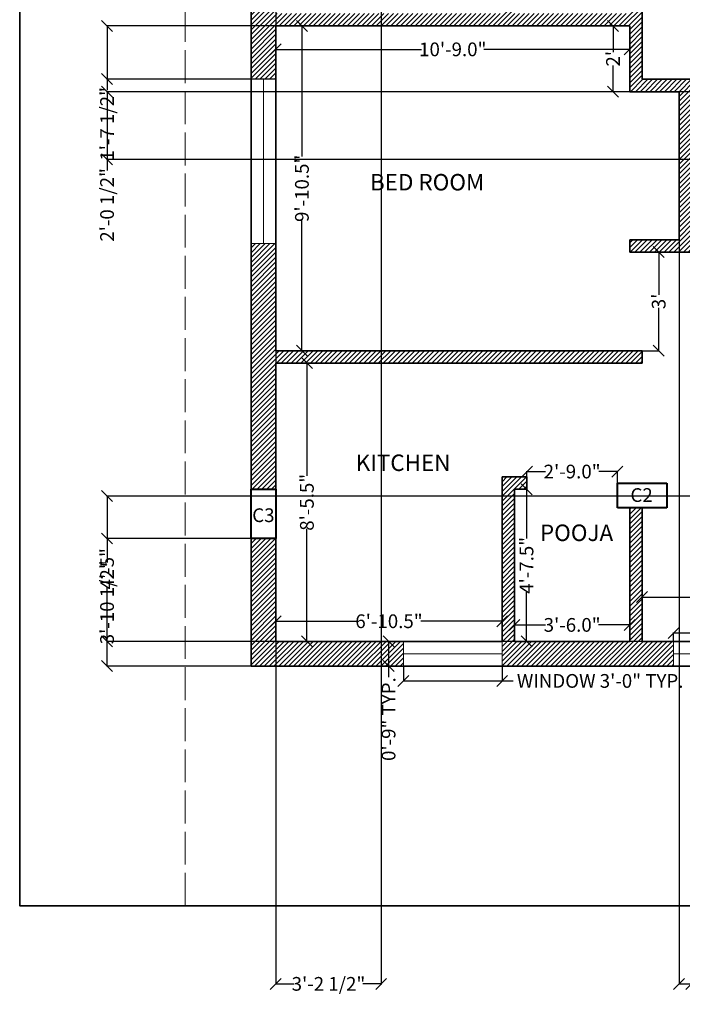
# Model space of a CAD drawing. Units: inches. Extents: x 72 to 538, y -43 to 598.
# Tile 1 of 4: x 72 to 314, y -43 to 316. Entities that reach past the tile are written whole.
import ezdxf

# ---------------------------------------------------------------- set-up
doc = ezdxf.new("R2010")
doc.units = ezdxf.units.IN
doc.header["$MEASUREMENT"] = 0
doc.linetypes.add('ACAD_ISO02W100', pattern=[15, 12, -3])
for name, color, linetype, lineweight in [('A-ANNO-DIMS', 2, 'Continuous', 18), ('A-ANNO-TEXT', 6, 'Continuous', 18), ('A-ANNO-TTLB', 7, 'Continuous', 35), ('A-AREA-IDEN', 7, 'Continuous', 25), ('A-COLS', 6, 'Continuous', 40), ('A-GLAZ', 4, 'Continuous', 18), ('A-WALL', 7, 'Continuous', 35), ('C-PROP', 3, 'ACAD_ISO02W100', 18)]:
    doc.layers.add(name, color=color, linetype=linetype, lineweight=lineweight)
doc.layers.add('A-WALL-PATT', color=30, linetype='Continuous', lineweight=13, true_color=0xf26722)
doc.styles.get("Standard").update_dxf_attribs({"font": 'arial.ttf'})
doc.dimstyles.get("Standard").update_dxf_attribs({"dimtxt": 5, "dimasz": 4, "dimexe": 0.18, "dimexo": 0.0625, "dimgap": 0.09, "dimtad": 0, "dimdec": 1, "dimzin": 0, "dimdsep": 46, "dimlunit": 3, "dimtxsty": 'Standard', "dimblk": 'OBLIQUE', "dimcen": 0.09, "dimadec": 0, "dimazin": 0, "dimtfac": 1, "dimtdec": 1, "dimtofl": 0, "dimtmove": 0, "dimatfit": 3, "dimfxl": 1, "dimtolj": 1, "dimtzin": 0, "dimarcsym": 0})

# ---------------------------------------------------------------- blocks, each defined once
blk = doc.blocks.new('_Oblique')
at = {"color": 0, "linetype": 'ByBlock', "lineweight": -2}
blk.add_line((-0.5, -0.5), (0.5, 0.5), dxfattribs=at)
blk = doc.blocks.new('*D11')
at = {"layer": 'A-ANNO-DIMS', "color": 0, "lineweight": -2, "transparency": 16777216}
for p, q in [((165.63, 313.56), (165.63, 304.87)), ((294.63, 313.56), (294.63, 304.87)), ((165.63, 305.05), (218.77, 305.05)), ((294.63, 305.05), (241.48, 305.05))]:
    blk.add_line(p, q, dxfattribs=at)
at = {"layer": 'Defpoints', "color": 0, "transparency": 16777216}
for p in [(165.63, 313.62), (294.63, 313.62), (294.63, 305.05)]:
    blk.add_point(p, dxfattribs=at)
at = {"layer": 'A-ANNO-DIMS', "color": 0, "lineweight": -2, "transparency": 16777216, "xscale": 4, "yscale": 4, "zscale": 4, "rotation": 180}
blk.add_blockref('_Oblique', (165.63, 305.05), dxfattribs=at)
at = {"layer": 'A-ANNO-DIMS', "color": 0, "lineweight": -2, "transparency": 16777216, "xscale": 4, "yscale": 4, "zscale": 4}
blk.add_blockref('_Oblique', (294.63, 305.05), dxfattribs=at)
at = {"layer": 'A-ANNO-DIMS', "color": 0, "transparency": 16777216, "insert": (230.13, 305.05), "char_height": 5, "attachment_point": 5}
blk.add_mtext('\\A1;10\'-9.0"', dxfattribs=at)
blk = doc.blocks.new('*D12')
at = {"layer": 'A-ANNO-DIMS', "color": 0, "lineweight": -2, "transparency": 16777216}
for p, q in [((294.57, 313.62), (288.36, 313.62)), ((288.54, 313.62), (288.54, 304.05)), ((288.54, 289.62), (288.54, 299.19)), ((294.57, 289.62), (288.36, 289.62))]:
    blk.add_line(p, q, dxfattribs=at)
at = {"layer": 'Defpoints', "color": 0, "transparency": 16777216}
for p in [(294.63, 313.62), (288.54, 289.62), (294.63, 289.62)]:
    blk.add_point(p, dxfattribs=at)
at = {"layer": 'A-ANNO-DIMS', "color": 0, "lineweight": -2, "transparency": 16777216, "xscale": 4, "yscale": 4, "zscale": 4}
for p, rotation in [((288.54, 313.62), 90), ((288.54, 289.62), 270)]:
    blk.add_blockref('_Oblique', p, dxfattribs=dict(at, rotation=rotation))
at = {"layer": 'A-ANNO-DIMS', "color": 0, "transparency": 16777216, "insert": (288.54, 301.62), "char_height": 5, "attachment_point": 5, "rotation": 90}
blk.add_mtext("\\A1;2'", dxfattribs=at)
blk = doc.blocks.new('*D13')
at = {"layer": 'A-ANNO-DIMS', "color": 0, "lineweight": -2, "transparency": 16777216}
for p, q in [((165.69, 313.62), (175.32, 313.62)), ((175.14, 313.62), (175.14, 265.96)), ((175.14, 195.12), (175.14, 242.78)), ((165.69, 195.12), (175.32, 195.12))]:
    blk.add_line(p, q, dxfattribs=at)
at = {"layer": 'Defpoints', "color": 0, "transparency": 16777216}
for p in [(165.63, 313.62), (165.63, 195.12), (175.14, 195.12)]:
    blk.add_point(p, dxfattribs=at)
at = {"layer": 'A-ANNO-DIMS', "color": 0, "lineweight": -2, "transparency": 16777216, "xscale": 4, "yscale": 4, "zscale": 4}
for p, rotation in [((175.14, 313.62), 90), ((175.14, 195.12), 270)]:
    blk.add_blockref('_Oblique', p, dxfattribs=dict(at, rotation=rotation))
at = {"layer": 'A-ANNO-DIMS', "color": 0, "transparency": 16777216, "insert": (175.14, 254.37), "char_height": 5, "attachment_point": 5, "rotation": 90}
blk.add_mtext('\\A1;9\'-10.5"', dxfattribs=at)
blk = doc.blocks.new('*D14')
at = {"layer": 'A-ANNO-DIMS', "color": 0, "lineweight": -2, "transparency": 16777216}
for p, q in [((165.69, 190.62), (177.14, 190.62)), ((176.96, 190.62), (176.96, 149.52)), ((176.96, 89.12), (176.96, 130.22)), ((165.69, 89.12), (177.14, 89.12))]:
    blk.add_line(p, q, dxfattribs=at)
at = {"layer": 'Defpoints', "color": 0, "transparency": 16777216}
for p in [(165.63, 190.62), (165.63, 89.12), (176.96, 89.12)]:
    blk.add_point(p, dxfattribs=at)
at = {"layer": 'A-ANNO-DIMS', "color": 0, "lineweight": -2, "transparency": 16777216, "xscale": 4, "yscale": 4, "zscale": 4}
for p, rotation in [((176.96, 190.62), 90), ((176.96, 89.12), 270)]:
    blk.add_blockref('_Oblique', p, dxfattribs=dict(at, rotation=rotation))
at = {"layer": 'A-ANNO-DIMS', "color": 0, "transparency": 16777216, "insert": (176.96, 139.87), "char_height": 5, "attachment_point": 5, "rotation": 90}
blk.add_mtext('\\A1;8\'-5.5"', dxfattribs=at)
blk = doc.blocks.new('*D15')
at = {"layer": 'A-ANNO-DIMS', "color": 0, "lineweight": -2, "transparency": 16777216}
for p, q in [((165.63, 89.18), (165.63, 96.67)), ((165.63, 96.49), (195.28, 96.49)), ((248.13, 96.49), (218.48, 96.49)), ((248.13, 89.18), (248.13, 96.67))]:
    blk.add_line(p, q, dxfattribs=at)
at = {"layer": 'Defpoints', "color": 0, "transparency": 16777216}
for p in [(248.13, 96.49), (165.63, 89.12), (248.13, 89.12)]:
    blk.add_point(p, dxfattribs=at)
at = {"layer": 'A-ANNO-DIMS', "color": 0, "lineweight": -2, "transparency": 16777216, "xscale": 4, "yscale": 4, "zscale": 4, "rotation": 180}
blk.add_blockref('_Oblique', (165.63, 96.49), dxfattribs=at)
at = {"layer": 'A-ANNO-DIMS', "color": 0, "lineweight": -2, "transparency": 16777216, "xscale": 4, "yscale": 4, "zscale": 4}
blk.add_blockref('_Oblique', (248.13, 96.49), dxfattribs=at)
at = {"layer": 'A-ANNO-DIMS', "color": 0, "transparency": 16777216, "insert": (206.88, 96.49), "char_height": 5, "attachment_point": 5}
blk.add_mtext('\\A1;6\'-10.5"', dxfattribs=at)
blk = doc.blocks.new('*D16')
at = {"layer": 'A-ANNO-DIMS', "color": 0, "lineweight": -2, "transparency": 16777216}
for p, q in [((252.63, 89.18), (252.63, 95.33)), ((252.63, 95.15), (263.98, 95.15)), ((294.63, 95.15), (283.28, 95.15)), ((294.63, 89.18), (294.63, 95.33))]:
    blk.add_line(p, q, dxfattribs=at)
at = {"layer": 'Defpoints', "color": 0, "transparency": 16777216}
for p in [(294.63, 95.15), (252.63, 89.12), (294.63, 89.12)]:
    blk.add_point(p, dxfattribs=at)
at = {"layer": 'A-ANNO-DIMS', "color": 0, "lineweight": -2, "transparency": 16777216, "xscale": 4, "yscale": 4, "zscale": 4, "rotation": 180}
blk.add_blockref('_Oblique', (252.63, 95.15), dxfattribs=at)
at = {"layer": 'A-ANNO-DIMS', "color": 0, "lineweight": -2, "transparency": 16777216, "xscale": 4, "yscale": 4, "zscale": 4}
blk.add_blockref('_Oblique', (294.63, 95.15), dxfattribs=at)
at = {"layer": 'A-ANNO-DIMS', "color": 0, "transparency": 16777216, "insert": (273.63, 95.15), "char_height": 5, "attachment_point": 5}
blk.add_mtext('\\A1;3\'-6.0"', dxfattribs=at)
blk = doc.blocks.new('*D17')
at = {"layer": 'A-ANNO-DIMS', "color": 0, "lineweight": -2, "transparency": 16777216}
for p, q in [((252.69, 144.62), (257.19, 144.62)), ((257.01, 144.62), (257.01, 126.62)), ((257.01, 89.12), (257.01, 107.12)), ((252.69, 89.12), (257.19, 89.12))]:
    blk.add_line(p, q, dxfattribs=at)
at = {"layer": 'Defpoints', "color": 0, "transparency": 16777216}
for p in [(252.63, 144.62), (252.63, 89.12), (257.01, 89.12)]:
    blk.add_point(p, dxfattribs=at)
at = {"layer": 'A-ANNO-DIMS', "color": 0, "lineweight": -2, "transparency": 16777216, "xscale": 4, "yscale": 4, "zscale": 4}
for p, rotation in [((257.01, 144.62), 90), ((257.01, 89.12), 270)]:
    blk.add_blockref('_Oblique', p, dxfattribs=dict(at, rotation=rotation))
at = {"layer": 'A-ANNO-DIMS', "color": 0, "transparency": 16777216, "insert": (257.01, 116.87), "char_height": 5, "attachment_point": 5, "rotation": 90}
blk.add_mtext('\\A1;4\'-7.5"', dxfattribs=at)
blk = doc.blocks.new('*D18')
at = {"layer": 'A-ANNO-DIMS', "color": 0, "lineweight": -2, "transparency": 16777216}
for p, q in [((257.13, 146.93), (257.13, 151.26)), ((257.13, 151.08), (263.94, 151.08)), ((290.13, 151.08), (283.32, 151.08)), ((290.13, 146.93), (290.13, 151.26))]:
    blk.add_line(p, q, dxfattribs=at)
at = {"layer": 'Defpoints', "color": 0, "transparency": 16777216}
for p in [(290.13, 151.08), (257.13, 146.87), (290.13, 146.87)]:
    blk.add_point(p, dxfattribs=at)
at = {"layer": 'A-ANNO-DIMS', "color": 0, "lineweight": -2, "transparency": 16777216, "xscale": 4, "yscale": 4, "zscale": 4, "rotation": 180}
blk.add_blockref('_Oblique', (257.13, 151.08), dxfattribs=at)
at = {"layer": 'A-ANNO-DIMS', "color": 0, "lineweight": -2, "transparency": 16777216, "xscale": 4, "yscale": 4, "zscale": 4}
blk.add_blockref('_Oblique', (290.13, 151.08), dxfattribs=at)
at = {"layer": 'A-ANNO-DIMS', "color": 0, "transparency": 16777216, "insert": (273.63, 151.08), "char_height": 5, "attachment_point": 5}
blk.add_mtext('\\A1;2\'-9.0"', dxfattribs=at)
blk = doc.blocks.new('*D19')
at = {"layer": 'A-ANNO-DIMS', "color": 0, "lineweight": -2, "transparency": 16777216}
for p, q in [((299.19, 231.12), (305.36, 231.12)), ((305.18, 231.12), (305.18, 215.51)), ((305.18, 195.12), (305.18, 210.73)), ((299.19, 195.12), (305.36, 195.12))]:
    blk.add_line(p, q, dxfattribs=at)
at = {"layer": 'Defpoints', "color": 0, "transparency": 16777216}
for p in [(299.13, 231.12), (305.18, 231.12), (299.13, 195.12)]:
    blk.add_point(p, dxfattribs=at)
at = {"layer": 'A-ANNO-DIMS', "color": 0, "lineweight": -2, "transparency": 16777216, "xscale": 4, "yscale": 4, "zscale": 4}
for p, rotation in [((305.18, 231.12), 90), ((305.18, 195.12), 270)]:
    blk.add_blockref('_Oblique', p, dxfattribs=dict(at, rotation=rotation))
at = {"layer": 'A-ANNO-DIMS', "color": 0, "transparency": 16777216, "insert": (305.18, 213.12), "char_height": 5, "attachment_point": 5, "rotation": 90}
blk.add_mtext("\\A1;3'", dxfattribs=at)
blk = doc.blocks.new('*D21')
at = {"layer": 'A-ANNO-DIMS', "color": 0, "lineweight": -2, "transparency": 16777216}
for p, q in [((299.13, 113.52), (299.13, 105.13)), ((441.63, 113.52), (441.63, 105.13)), ((299.13, 105.31), (357.08, 105.31)), ((441.63, 105.31), (383.68, 105.31))]:
    blk.add_line(p, q, dxfattribs=at)
at = {"layer": 'Defpoints', "color": 0, "transparency": 16777216}
for p in [(299.13, 113.59), (441.63, 113.59), (441.63, 105.31)]:
    blk.add_point(p, dxfattribs=at)
at = {"layer": 'A-ANNO-DIMS', "color": 0, "lineweight": -2, "transparency": 16777216, "xscale": 4, "yscale": 4, "zscale": 4, "rotation": 180}
blk.add_blockref('_Oblique', (299.13, 105.31), dxfattribs=at)
at = {"layer": 'A-ANNO-DIMS', "color": 0, "lineweight": -2, "transparency": 16777216, "xscale": 4, "yscale": 4, "zscale": 4}
blk.add_blockref('_Oblique', (441.63, 105.31), dxfattribs=at)
at = {"layer": 'A-ANNO-DIMS', "color": 0, "transparency": 16777216, "insert": (370.38, 105.31), "char_height": 5, "attachment_point": 5}
blk.add_mtext('\\A1;11\'-10.5"', dxfattribs=at)
blk = doc.blocks.new('*D36')
at = {"layer": 'A-ANNO-DIMS', "color": 0, "lineweight": -2, "transparency": 16777216}
for p, q in [((310.61, 89.18), (310.61, 92.39)), ((310.61, 92.21), (338.22, 92.21)), ((370.61, 92.21), (343, 92.21)), ((370.61, 89.18), (370.61, 92.39))]:
    blk.add_line(p, q, dxfattribs=at)
at = {"layer": 'Defpoints', "color": 0, "transparency": 16777216}
for p in [(370.61, 92.21), (310.61, 89.12), (370.61, 89.12)]:
    blk.add_point(p, dxfattribs=at)
at = {"layer": 'A-ANNO-DIMS', "color": 0, "lineweight": -2, "transparency": 16777216, "xscale": 4, "yscale": 4, "zscale": 4, "rotation": 180}
blk.add_blockref('_Oblique', (310.61, 92.21), dxfattribs=at)
at = {"layer": 'A-ANNO-DIMS', "color": 0, "lineweight": -2, "transparency": 16777216, "xscale": 4, "yscale": 4, "zscale": 4}
blk.add_blockref('_Oblique', (370.61, 92.21), dxfattribs=at)
at = {"layer": 'A-ANNO-DIMS', "color": 0, "transparency": 16777216, "insert": (340.61, 92.21), "char_height": 5, "attachment_point": 5}
blk.add_mtext("\\A1;5'", dxfattribs=at)
blk = doc.blocks.new('COL-9X18')
for p, q in [((0, 18), (9, 18)), ((0, 0), (0, 18)), ((9, 18), (9, 0)), ((9, 0), (0, 0))]:
    blk.add_line(p, q)
blk = doc.blocks.new('WIN-60')
for p, q in [((0, 9), (0, 0)), ((60, 9), (60, 0)), ((0, 4.5), (60, 4.5))]:
    blk.add_line(p, q)
blk = doc.blocks.new('WIN-36')
for p, q in [((9, 36), (0, 36)), ((4.5, 36), (4.5, 0)), ((9, 0), (0, 0))]:
    blk.add_line(p, q)
blk = doc.blocks.new('*D48')
at = {"layer": 'A-ANNO-DIMS', "color": 0, "lineweight": -2, "transparency": 16777216}
for p, q in [((212.13, 80.06), (212.13, 74.54)), ((248.13, 80.06), (248.13, 74.54)), ((212.13, 74.72), (248.13, 74.72)), ((248.13, 74.72), (252.13, 74.72))]:
    blk.add_line(p, q, dxfattribs=at)
at = {"layer": 'Defpoints', "color": 0, "transparency": 16777216}
for p in [(212.13, 80.12), (248.13, 80.12), (248.13, 74.72)]:
    blk.add_point(p, dxfattribs=at)
at = {"layer": 'A-ANNO-DIMS', "color": 0, "lineweight": -2, "transparency": 16777216, "xscale": 4, "yscale": 4, "zscale": 4, "rotation": 180}
blk.add_blockref('_Oblique', (212.13, 74.72), dxfattribs=at)
at = {"layer": 'A-ANNO-DIMS', "color": 0, "lineweight": -2, "transparency": 16777216, "xscale": 4, "yscale": 4, "zscale": 4}
blk.add_blockref('_Oblique', (248.13, 74.72), dxfattribs=at)
at = {"layer": 'A-ANNO-DIMS', "color": 0, "transparency": 16777216, "insert": (283.85, 74.72), "char_height": 5, "attachment_point": 5}
blk.add_mtext('\\A1;WINDOW 3\'-0" TYP.', dxfattribs=at)
blk = doc.blocks.new('*D49')
at = {"layer": 'A-ANNO-DIMS', "color": 0, "lineweight": -2, "transparency": 16777216}
for p, q in [((212.07, 89.12), (206.55, 89.12)), ((206.73, 89.12), (206.73, 80.12)), ((212.07, 80.12), (206.55, 80.12)), ((206.73, 80.12), (206.73, 76.12))]:
    blk.add_line(p, q, dxfattribs=at)
at = {"layer": 'Defpoints', "color": 0, "transparency": 16777216}
for p in [(212.13, 89.12), (206.73, 80.12), (212.13, 80.12)]:
    blk.add_point(p, dxfattribs=at)
at = {"layer": 'A-ANNO-DIMS', "color": 0, "lineweight": -2, "transparency": 16777216, "xscale": 4, "yscale": 4, "zscale": 4}
for p, rotation in [((206.73, 89.12), 90), ((206.73, 80.12), 270)]:
    blk.add_blockref('_Oblique', p, dxfattribs=dict(at, rotation=rotation))
at = {"layer": 'A-ANNO-DIMS', "color": 0, "transparency": 16777216, "insert": (206.73, 60.79), "char_height": 5, "attachment_point": 5, "rotation": 90}
blk.add_mtext('\\A1;0\'-9" TYP.', dxfattribs=at)
blk = doc.blocks.new('*D57')
at = {"layer": 'A-ANNO-DIMS', "color": 0, "lineweight": -2, "transparency": 16777216}
for p, q in [((165.63, 527.06), (165.63, -35.94)), ((204.03, 527.06), (204.03, -35.94)), ((165.63, -35.76), (172.27, -35.76)), ((204.03, -35.76), (197.39, -35.76))]:
    blk.add_line(p, q, dxfattribs=at)
at = {"layer": 'Defpoints', "color": 0, "transparency": 16777216}
for p in [(165.63, 527.12), (204.03, 527.12), (204.03, -35.76)]:
    blk.add_point(p, dxfattribs=at)
at = {"layer": 'A-ANNO-DIMS', "color": 0, "lineweight": -2, "transparency": 16777216, "xscale": 4, "yscale": 4, "zscale": 4, "rotation": 180}
blk.add_blockref('_Oblique', (165.63, -35.76), dxfattribs=at)
at = {"layer": 'A-ANNO-DIMS', "color": 0, "lineweight": -2, "transparency": 16777216, "xscale": 4, "yscale": 4, "zscale": 4}
blk.add_blockref('_Oblique', (204.03, -35.76), dxfattribs=at)
at = {"layer": 'A-ANNO-DIMS', "color": 0, "transparency": 16777216, "insert": (184.83, -35.76), "char_height": 5, "attachment_point": 5}
blk.add_mtext('\\A1;3\'-2 1/2"', dxfattribs=at)
blk = doc.blocks.new('*D59')
at = {"layer": 'A-ANNO-DIMS', "color": 0, "lineweight": -2, "transparency": 16777216}
for p, q in [((165.57, 313.62), (103.95, 313.62)), ((104.13, 313.62), (104.13, 294.2)), ((165.57, 294.2), (103.95, 294.2)), ((104.13, 294.2), (104.13, 290.2))]:
    blk.add_line(p, q, dxfattribs=at)
at = {"layer": 'Defpoints', "color": 0, "transparency": 16777216}
for p in [(165.63, 313.62), (104.13, 294.2), (165.63, 294.2)]:
    blk.add_point(p, dxfattribs=at)
at = {"layer": 'A-ANNO-DIMS', "color": 0, "lineweight": -2, "transparency": 16777216, "xscale": 4, "yscale": 4, "zscale": 4}
for p, rotation in [((104.13, 313.62), 90), ((104.13, 294.2), 270)]:
    blk.add_blockref('_Oblique', p, dxfattribs=dict(at, rotation=rotation))
at = {"layer": 'A-ANNO-DIMS', "color": 0, "transparency": 16777216, "insert": (104.13, 277.88), "char_height": 5, "attachment_point": 5, "rotation": 90}
blk.add_mtext('\\A1;1\'-7 1/2"', dxfattribs=at)
blk = doc.blocks.new('*D65')
at = {"layer": 'A-ANNO-DIMS', "color": 0, "lineweight": -2, "transparency": 16777216}
for p, q in [((312.63, 235.56), (312.63, -35.94)), ((317.13, 231.06), (317.13, -35.94)), ((312.63, -35.76), (317.13, -35.76)), ((317.13, -35.76), (321.13, -35.76))]:
    blk.add_line(p, q, dxfattribs=at)
at = {"layer": 'Defpoints', "color": 0, "transparency": 16777216}
for p in [(312.63, 235.62), (317.13, 231.12), (317.13, -35.76)]:
    blk.add_point(p, dxfattribs=at)
at = {"layer": 'A-ANNO-DIMS', "color": 0, "lineweight": -2, "transparency": 16777216, "xscale": 4, "yscale": 4, "zscale": 4, "rotation": 180}
blk.add_blockref('_Oblique', (312.63, -35.76), dxfattribs=at)
at = {"layer": 'A-ANNO-DIMS', "color": 0, "lineweight": -2, "transparency": 16777216, "xscale": 4, "yscale": 4, "zscale": 4}
blk.add_blockref('_Oblique', (317.13, -35.76), dxfattribs=at)
at = {"layer": 'A-ANNO-DIMS', "color": 0, "transparency": 16777216, "insert": (333.69, -35.76), "char_height": 5, "attachment_point": 5}
blk.add_mtext('\\A1;0\'-4 1/2"', dxfattribs=at)
blk = doc.blocks.new('*D66')
at = {"layer": 'A-ANNO-DIMS', "color": 0, "lineweight": -2, "transparency": 16777216}
for p, q in [((441.57, 289.62), (103.95, 289.62)), ((104.13, 289.62), (104.13, 264.93)), ((441.57, 264.93), (103.95, 264.93)), ((104.13, 264.93), (104.13, 260.93))]:
    blk.add_line(p, q, dxfattribs=at)
at = {"layer": 'Defpoints', "color": 0, "transparency": 16777216}
for p in [(441.63, 289.62), (104.13, 264.93), (441.63, 264.93)]:
    blk.add_point(p, dxfattribs=at)
at = {"layer": 'A-ANNO-DIMS', "color": 0, "lineweight": -2, "transparency": 16777216, "xscale": 4, "yscale": 4, "zscale": 4}
for p, rotation in [((104.13, 289.62), 90), ((104.13, 264.93), 270)]:
    blk.add_blockref('_Oblique', p, dxfattribs=dict(at, rotation=rotation))
at = {"layer": 'A-ANNO-DIMS', "color": 0, "transparency": 16777216, "insert": (104.13, 248.33), "char_height": 5, "attachment_point": 5, "rotation": 90}
blk.add_mtext('\\A1;2\'-0 1/2"', dxfattribs=at)
blk = doc.blocks.new('*D67')
at = {"layer": 'A-ANNO-DIMS', "color": 0, "lineweight": -2, "transparency": 16777216}
for p, q in [((156.57, 126.66), (103.95, 126.66)), ((104.13, 126.66), (104.13, 117.89)), ((104.13, 80.12), (104.13, 88.89)), ((156.57, 80.12), (103.95, 80.12))]:
    blk.add_line(p, q, dxfattribs=at)
at = {"layer": 'Defpoints', "color": 0, "transparency": 16777216}
for p in [(156.63, 126.66), (104.13, 80.12), (156.63, 80.12)]:
    blk.add_point(p, dxfattribs=at)
at = {"layer": 'A-ANNO-DIMS', "color": 0, "lineweight": -2, "transparency": 16777216, "xscale": 4, "yscale": 4, "zscale": 4}
for p, rotation in [((104.13, 126.66), 90), ((104.13, 80.12), 270)]:
    blk.add_blockref('_Oblique', p, dxfattribs=dict(at, rotation=rotation))
at = {"layer": 'A-ANNO-DIMS', "color": 0, "transparency": 16777216, "insert": (104.13, 103.39), "char_height": 5, "attachment_point": 5, "rotation": 90}
blk.add_mtext('\\A1;3\'-10 1/2"', dxfattribs=at)
blk = doc.blocks.new('*D69')
at = {"layer": 'A-ANNO-DIMS', "color": 0, "lineweight": -2, "transparency": 16777216}
for p, q in [((441.57, 142.12), (103.95, 142.12)), ((104.13, 142.12), (104.13, 122.46)), ((104.13, 89.12), (104.13, 108.78)), ((441.57, 89.12), (103.95, 89.12))]:
    blk.add_line(p, q, dxfattribs=at)
at = {"layer": 'Defpoints', "color": 0, "transparency": 16777216}
for p in [(441.63, 142.12), (104.13, 89.12), (441.63, 89.12)]:
    blk.add_point(p, dxfattribs=at)
at = {"layer": 'A-ANNO-DIMS', "color": 0, "lineweight": -2, "transparency": 16777216, "xscale": 4, "yscale": 4, "zscale": 4}
for p, rotation in [((104.13, 142.12), 90), ((104.13, 89.12), 270)]:
    blk.add_blockref('_Oblique', p, dxfattribs=dict(at, rotation=rotation))
at = {"layer": 'A-ANNO-DIMS', "color": 0, "transparency": 16777216, "insert": (104.13, 115.62), "char_height": 5, "attachment_point": 5, "rotation": 90}
blk.add_mtext('\\A1;4\'-5"', dxfattribs=at)

msp = doc.modelspace()

# ---------------------------------------------------------------- hatches: boundary and pattern name
at = {"layer": 'A-WALL-PATT'}
h = msp.add_hatch(dxfattribs=at)
h.set_pattern_fill('ANSI31', color=256, scale=10)
h.paths.add_polyline_path([(204.03, 536.12), (165.63, 536.12), (165.63, 527.12), (204.03, 527.12)])
h.paths.add_polyline_path([(165.63, 487.18), (165.63, 518.12), (156.63, 518.12), (156.63, 487.18)])
h.paths.add_polyline_path([(374.85, 253.74), (416.04, 253.74), (416.04, 266.11), (374.85, 266.11)], flags=9)
h.paths.add_polyline_path([(358.05, 165.41), (382.02, 165.41), (382.02, 177.78), (358.05, 177.78)], flags=9)
h.paths.add_polyline_path([(258.82, 340.82), (290.25, 340.82), (290.25, 353.18), (258.82, 353.18)], flags=9)
h.paths.add_polyline_path([(190.8, 385.39), (230.59, 385.39), (230.59, 397.75), (190.8, 397.75)], flags=9)
h.paths.add_polyline_path([(259.76, 122.35), (291.18, 122.35), (291.18, 134.72), (259.76, 134.72)], flags=9)
h.paths.add_polyline_path([(192.66, 147.9), (232.45, 147.9), (232.45, 160.26), (192.66, 160.26)], flags=9)
h.paths.add_polyline_path([(197.84, 250.21), (246.48, 250.21), (246.48, 262.58), (197.84, 262.58)], flags=9)
h.paths.add_polyline_path([(329.22, 365.75), (353.18, 365.75), (353.18, 378.11), (329.22, 378.11)], flags=9)
h.paths.add_polyline_path([(351.21, 489.41), (392.39, 489.41), (392.39, 501.77), (351.21, 501.77)], flags=9)
h.paths.add_polyline_path([(193.31, 469.76), (241.95, 469.76), (241.95, 482.12), (193.31, 482.12)], flags=9)
h.paths.add_polyline_path([(262.62, 413.67), (274.04, 413.67), (274.04, 423.97), (262.62, 423.97)], flags=9)
h.paths.add_polyline_path([(155.57, 341.76), (167, 341.76), (167, 352.06), (155.57, 352.06)], flags=9)
h.paths.add_polyline_path([(155.43, 129.83), (166.86, 129.83), (166.86, 140.14), (155.43, 140.14)], flags=9)
h.paths.add_polyline_path([(293.27, 137.19), (304.7, 137.19), (304.7, 147.49), (293.27, 147.49)], flags=9)
h.paths.add_polyline_path([(440.6, 145.74), (452.03, 145.74), (452.03, 156.04), (440.6, 156.04)], flags=9)
h.paths.add_polyline_path([(422.43, 340.03), (433.86, 340.03), (433.86, 350.33), (422.43, 350.33)], flags=9)
h.paths.add_polyline_path([(155.47, 520.54), (166.9, 520.54), (166.9, 530.84), (155.47, 530.84)], flags=9)
h.paths.add_polyline_path([(348.1, 449.93), (374.22, 449.93), (374.22, 460.24), (348.1, 460.24)], flags=9)
h.paths.add_polyline_path([(417.29, 368.09), (417.29, 394.21), (406.99, 394.21), (406.99, 368.09)], flags=9)
h.paths.add_polyline_path([(422.51, 520.96), (433.94, 520.96), (433.94, 531.26), (422.51, 531.26)], flags=9)
h.paths.add_polyline_path([(284.05, 526.61), (295.48, 526.61), (295.48, 536.92), (284.05, 536.92)], flags=9)
h = msp.add_hatch(dxfattribs=at)
h.set_pattern_fill('ANSI31', color=256, scale=10)
h.paths.add_polyline_path([(432.63, 468.62), (432.63, 518.12), (423.63, 518.12), (423.63, 473.12), (339.63, 473.12), (335.13, 473.12), (335.13, 468.62), (423.63, 468.62), (423.63, 354.62), (432.63, 354.62)])
h.paths.add_polyline_path([(450.63, 231.12), (450.63, 240.93), (441.63, 240.93), (441.63, 235.62), (357.63, 235.62), (353.13, 235.62), (353.13, 231.12), (441.63, 231.12)])
h.paths.add_polyline_path([(374.85, 253.74), (416.04, 253.74), (416.04, 266.11), (374.85, 266.11)], flags=9)
h.paths.add_polyline_path([(358.05, 165.41), (382.02, 165.41), (382.02, 177.78), (358.05, 177.78)], flags=9)
h.paths.add_polyline_path([(258.82, 340.82), (290.25, 340.82), (290.25, 353.18), (258.82, 353.18)], flags=9)
h.paths.add_polyline_path([(190.8, 385.39), (230.59, 385.39), (230.59, 397.75), (190.8, 397.75)], flags=9)
h.paths.add_polyline_path([(259.76, 122.35), (291.18, 122.35), (291.18, 134.72), (259.76, 134.72)], flags=9)
h.paths.add_polyline_path([(192.66, 147.9), (232.45, 147.9), (232.45, 160.26), (192.66, 160.26)], flags=9)
h.paths.add_polyline_path([(197.84, 250.21), (246.48, 250.21), (246.48, 262.58), (197.84, 262.58)], flags=9)
h.paths.add_polyline_path([(329.22, 365.75), (353.18, 365.75), (353.18, 378.11), (329.22, 378.11)], flags=9)
h.paths.add_polyline_path([(351.21, 489.41), (392.39, 489.41), (392.39, 501.77), (351.21, 501.77)], flags=25)
h.paths.add_polyline_path([(193.31, 469.76), (241.95, 469.76), (241.95, 482.12), (193.31, 482.12)], flags=9)
h.paths.add_polyline_path([(262.62, 413.67), (274.04, 413.67), (274.04, 423.97), (262.62, 423.97)], flags=9)
h.paths.add_polyline_path([(155.57, 341.76), (167, 341.76), (167, 352.06), (155.57, 352.06)], flags=9)
h.paths.add_polyline_path([(155.43, 129.83), (166.86, 129.83), (166.86, 140.14), (155.43, 140.14)], flags=9)
h.paths.add_polyline_path([(293.27, 137.19), (304.7, 137.19), (304.7, 147.49), (293.27, 147.49)], flags=9)
h.paths.add_polyline_path([(440.6, 145.74), (452.03, 145.74), (452.03, 156.04), (440.6, 156.04)], flags=9)
h.paths.add_polyline_path([(422.43, 340.03), (433.86, 340.03), (433.86, 350.33), (422.43, 350.33)], flags=9)
h.paths.add_polyline_path([(422.51, 520.96), (433.94, 520.96), (433.94, 531.26), (422.51, 531.26)], flags=9)
h.paths.add_polyline_path([(284.05, 526.61), (295.48, 526.61), (295.48, 536.92), (284.05, 536.92)], flags=9)
h.paths.add_polyline_path([(155.47, 520.54), (166.9, 520.54), (166.9, 530.84), (155.47, 530.84)], flags=9)
h = msp.add_hatch(dxfattribs=at)
h.set_pattern_fill('ANSI31', color=256, scale=10)
h.paths.add_polyline_path([(165.63, 427.18), (156.63, 427.18), (156.63, 414.62), (165.63, 414.62), (258.91, 414.62), (258.91, 419.12), (165.63, 419.12)])
h.paths.add_polyline_path([(165.63, 378.62), (156.63, 378.62), (156.63, 355.53), (165.63, 355.53)])
h.paths.add_polyline_path([(299.13, 378.12), (290.13, 378.12), (290.13, 373.62), (294.63, 373.62), (294.63, 318.12), (252.63, 318.12), (252.63, 373.62), (257.13, 373.62), (257.13, 378.12), (248.13, 378.12), (248.13, 318.12), (165.63, 318.12), (165.63, 337.53), (156.63, 337.53), (156.63, 294.2), (165.63, 294.2), (165.63, 313.62), (294.63, 313.62), (294.63, 289.62), (312.63, 289.62), (312.63, 235.62), (294.63, 235.62), (294.63, 231.12), (317.13, 231.12), (317.13, 289.62), (353.13, 289.62), (353.13, 265.62), (357.63, 265.62), (357.63, 289.62), (441.63, 289.62), (441.63, 264.93), (450.63, 264.93), (450.63, 294.12), (432.63, 294.12), (299.13, 294.12)])
h.paths.add_polyline_path([(299.13, 195.12), (165.63, 195.12), (165.63, 234.2), (156.63, 234.2), (156.63, 144.66), (165.63, 144.66), (165.63, 190.62), (299.13, 190.62)])
h.paths.add_polyline_path([(165.63, 126.66), (156.63, 126.66), (156.63, 80.12), (212.13, 80.12), (212.13, 89.12), (165.63, 89.12)])
h.paths.add_polyline_path([(310.61, 89.12), (299.13, 89.12), (299.13, 137.87), (294.63, 137.87), (294.63, 89.12), (252.63, 89.12), (252.63, 144.62), (257.13, 144.62), (257.13, 149.12), (248.13, 149.12), (248.13, 89.12), (248.13, 80.12), (310.61, 80.12)])
h.paths.add_polyline_path([(450.63, 142.12), (441.63, 142.12), (441.63, 89.12), (433.82, 89.12), (433.82, 80.12), (450.63, 80.12)])
h.paths.add_polyline_path([(450.63, 171.12), (446.13, 171.12), (441.63, 171.12), (441.63, 160.12), (450.63, 160.12)])
h.paths.add_polyline_path([(281.13, 536.12), (264.03, 536.12), (264.03, 527.12), (281.13, 527.12)])
h.paths.add_polyline_path([(339.63, 536.12), (299.13, 536.12), (299.13, 527.12), (335.13, 527.12), (335.13, 503.12), (339.63, 503.12), (339.63, 527.12)])
h.paths.add_polyline_path([(299.13, 527.12), (294.63, 527.12), (294.63, 455.12), (299.13, 455.12)])
h.paths.add_polyline_path([(492.63, 536.12), (432.63, 536.12), (432.63, 527.12), (492.63, 527.12)])
h.paths.add_polyline_path([(423.63, 536.12), (363.63, 536.12), (363.63, 527.12), (423.63, 527.12)])
h.paths.add_polyline_path([(299.13, 419.12), (276.91, 419.12), (276.91, 414.62), (299.13, 414.62)])

# ---------------------------------------------------------------- linework, layer by layer
at = {"layer": 'A-ANNO-TTLB'}
msp.add_lwpolyline([(72.29, 598.2), (537.75, 598.2), (537.75, -7.26), (72.29, -7.26)], close=True, dxfattribs=at)
at = {"layer": 'A-WALL'}
for p, q in [((156.63, 80.12), (156.63, 536.12)), ((299.13, 294.12), (299.13, 378.12)), ((165.63, 313.62), (294.63, 313.62)), ((165.63, 195.12), (165.63, 313.62)), ((294.63, 313.62), (294.63, 289.62)), ((299.13, 294.12), (432.63, 294.12)), ((294.63, 289.62), (312.63, 289.62)), ((294.63, 289.62), (312.63, 289.62)), ((312.63, 289.62), (312.63, 235.62)), ((294.63, 235.62), (312.63, 235.62)), ((294.63, 231.12), (294.63, 235.62)), ((294.63, 231.12), (317.13, 231.12)), ((165.63, 195.12), (299.13, 195.12)), ((299.13, 190.62), (299.13, 195.12)), ((165.63, 89.12), (165.63, 190.62)), ((165.63, 190.62), (299.13, 190.62)), ((248.13, 89.12), (248.13, 149.12)), ((257.13, 149.12), (248.13, 149.12)), ((248.13, 149.12), (257.13, 149.12)), ((257.13, 149.12), (257.13, 144.62)), ((252.63, 89.12), (252.63, 144.62)), ((257.13, 144.62), (252.63, 144.62)), ((294.63, 89.12), (294.63, 138.05)), ((299.13, 89.12), (299.13, 138.05)), ((248.13, 89.12), (165.63, 89.12)), ((294.63, 89.12), (252.63, 89.12)), ((391.82, 89.12), (299.13, 89.12)), ((391.82, 80.12), (156.63, 80.12))]:
    msp.add_line(p, q, dxfattribs=at)
at = {"layer": 'C-PROP'}
msp.add_line((132.63, -7.26), (132.63, 560.12), dxfattribs=at)

# ---------------------------------------------------------------- block references
at = {"layer": 'A-COLS'}
msp.add_blockref('COL-9X18', (156.63, 126.66), dxfattribs=at)
at = {"layer": 'A-COLS', "rotation": 90.00000000000043}
msp.add_blockref('COL-9X18', (308.13, 137.87), dxfattribs=at)
at = {"layer": 'A-GLAZ'}
for name, p, rotation in [('WIN-60', (156.63, 294.2), 269.9999999999998), ('WIN-36', (212.13, 89.12), 270), ('WIN-60', (370.61, 89.12), 180)]:
    msp.add_blockref(name, p, dxfattribs=dict(at, rotation=rotation))

# ---------------------------------------------------------------- texts
at = {"layer": 'A-ANNO-TEXT', "char_height": 5, "attachment_point": 1}
for s, insert in [('C2', (294.87, 145)), ('C3', (157.03, 137.65))]:
    msp.add_mtext_dynamic_manual_height_columns(s, width=12, gutter_width=1, heights=[0], dxfattribs=dict(at, insert=insert))
at = {"layer": 'A-AREA-IDEN', "char_height": 6, "attachment_point": 1}
for s, insert in [('BED ROOM', (199.95, 259.6)), ('KITCHEN', (194.77, 157.28)), ('POOJA', (261.9, 131.74))]:
    msp.add_mtext_dynamic_manual_height_columns(s, width=78.4308, gutter_width=1, heights=[0], dxfattribs=dict(at, insert=insert))

# ---------------------------------------------------------------- dimensions: what is measured, and where the dimension line sits
at = {"layer": 'A-ANNO-DIMS'}
for base, p1, p2, override, picture, middle in [((204.03, -35.76), (165.63, 527.12), (204.03, 527.12), {"dimdec": 1, "dimlfac": 1, "dimrnd": 0, "dimzin": 1, "dimdsep": 46, "dimlunit": 4, "dimfrac": 2}, '*D57', (184.83, -35.76)), ((294.63, 305.05), (165.63, 313.62), (294.63, 313.62), {"dimclrd": 0, "dimclre": 0, "dimclrt": 0}, '*D11', (230.13, 305.05)), ((317.13, -35.76), (312.63, 235.62), (317.13, 231.12), {"dimdec": 1, "dimlfac": 1, "dimrnd": 0, "dimzin": 1, "dimdsep": 46, "dimlunit": 4, "dimfrac": 2}, '*D65', (333.69, -35.76)), ((290.13, 151.08), (257.13, 146.87), (290.13, 146.87), {"dimclrd": 0, "dimclre": 0, "dimclrt": 0}, '*D18', (273.63, 151.08)), ((441.63, 105.31), (299.13, 113.59), (441.63, 113.59), {"dimclrd": 0, "dimclre": 0, "dimclrt": 0}, '*D21', (370.38, 105.31)), ((248.13, 96.49), (165.63, 89.12), (248.13, 89.12), {"dimclrd": 0, "dimclre": 0, "dimclrt": 0}, '*D15', (206.88, 96.49)), ((294.63, 95.15), (252.63, 89.12), (294.63, 89.12), {"dimclrd": 0, "dimclre": 0, "dimclrt": 0}, '*D16', (273.63, 95.15)), ((370.61, 92.21), (310.61, 89.12), (370.61, 89.12), {"dimclrd": 0, "dimclre": 0, "dimclrt": 0}, '*D36', (340.61, 92.21))]:
    dim = msp.add_linear_dim(base=base, p1=p1, p2=p2, dimstyle='Standard', override=override, dxfattribs=at)
    dim.commit()
    dim.dimension.update_dxf_attribs({"geometry": picture, "text_midpoint": middle})
for base, p1, p2, override, picture, middle in [((104.13, 294.2), (165.63, 313.62), (165.63, 294.2), {"dimdec": 1, "dimlfac": 1, "dimrnd": 0, "dimzin": 1, "dimdsep": 46, "dimlunit": 4, "dimfrac": 2}, '*D59', (104.13, 277.88)), ((175.14, 195.12), (165.63, 313.62), (165.63, 195.12), {"dimclrd": 0, "dimclre": 0, "dimclrt": 0}, '*D13', (175.14, 254.37)), ((288.54, 289.62), (294.63, 313.62), (294.63, 289.62), {"dimclrd": 0, "dimclre": 0, "dimclrt": 0}, '*D12', (288.54, 301.62)), ((104.13, 264.93), (441.63, 289.62), (441.63, 264.93), {"dimdec": 1, "dimlfac": 1, "dimrnd": 0, "dimzin": 1, "dimdsep": 46, "dimlunit": 4, "dimfrac": 2}, '*D66', (104.13, 248.33)), ((305.18, 231.12), (299.13, 195.12), (299.13, 231.12), {"dimclrd": 0, "dimclre": 0, "dimclrt": 0}, '*D19', (305.18, 213.12)), ((176.96, 89.12), (165.63, 190.62), (165.63, 89.12), {"dimclrd": 0, "dimclre": 0, "dimclrt": 0}, '*D14', (176.96, 139.87)), ((104.13, 89.12), (441.63, 142.12), (441.63, 89.12), {"dimdec": 1, "dimlfac": 1, "dimrnd": 0, "dimzin": 1, "dimdsep": 46, "dimlunit": 4, "dimfrac": 2}, '*D69', (104.13, 115.62)), ((257.01, 89.12), (252.63, 144.62), (252.63, 89.12), {"dimclrd": 0, "dimclre": 0, "dimclrt": 0}, '*D17', (257.01, 116.87)), ((104.13, 80.12), (156.63, 126.66), (156.63, 80.12), {"dimdec": 1, "dimlfac": 1, "dimrnd": 0, "dimzin": 1, "dimdsep": 46, "dimlunit": 4, "dimfrac": 2}, '*D67', (104.13, 103.39))]:
    dim = msp.add_linear_dim(base=base, p1=p1, p2=p2, angle=90, dimstyle='Standard', override=override, dxfattribs=at)
    dim.commit()
    dim.dimension.update_dxf_attribs({"geometry": picture, "text_midpoint": middle})
dim = msp.add_linear_dim(base=(206.73, 80.12), p1=(212.13, 89.12), p2=(212.13, 80.12), angle=270, text='<> TYP.', dimstyle='Standard', override={"dimdec": 1, "dimlfac": 1, "dimrnd": 0, "dimzin": 1, "dimdsep": 46, "dimlunit": 4, "dimfrac": 2}, dxfattribs=at)
dim.commit()
dim.dimension.update_dxf_attribs({"geometry": '*D49', "text_midpoint": (206.73, 60.79)})
dim = msp.add_linear_dim(base=(248.13, 74.72), p1=(212.13, 80.12), p2=(248.13, 80.12), text='WINDOW <> TYP.', dimstyle='Standard', override={"dimdec": 1, "dimlfac": 1, "dimrnd": 0, "dimzin": 1, "dimdsep": 46, "dimlunit": 4, "dimfrac": 2}, dxfattribs=at)
dim.commit()
dim.dimension.update_dxf_attribs({"geometry": '*D48', "text_midpoint": (283.85, 74.72)})

doc.saveas('drawing.dxf')
